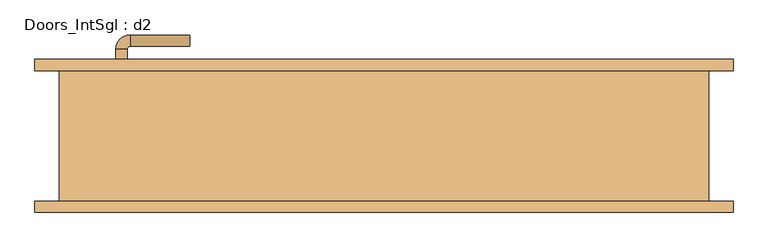
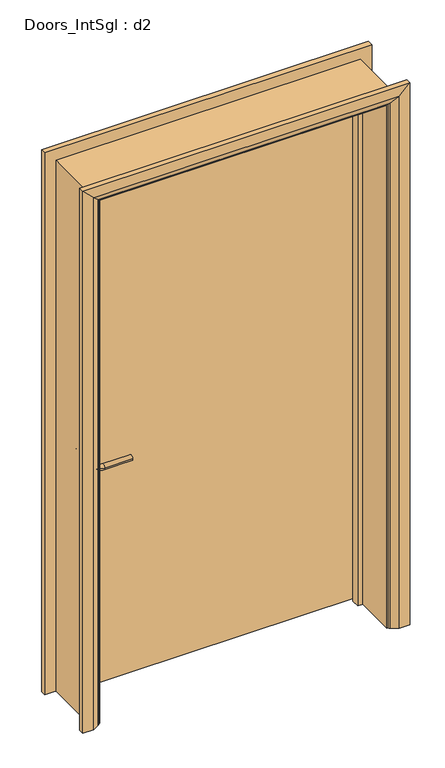
"""IFC4 building model written with IfcOpenShell, lengths in millimetres: door geometry, Doors_IntSgl : d2."""

from ifc_helpers import new_model, si_unit, point, frame, frame_2d, origin, place, context, project, spatial, polyline, circle_curve, ellipse_curve, trimmed, segment, composite_curve, outline, extrude, faceted_brep, source, transform, mapped, element, save
from ifc_brep_helpers import plane_surface, cylinder_surface, revolved_surface, advanced_brep


def doors_intsgl_d2_d6dd0e7a(model_context):
    return source(origin(), model_context, "Body", "SolidModel", [
        advanced_brep(
        [(-470.85, 68.3, 900.0), (-450.85, 68.3, 900.0), (-450.85, 38.3, 900.0), (-470.85, 38.3, 900.0), (-445.85, 33.3, 900.0), (-445.85, 13.3, 900.0), (-340.85, 13.3, 900.0), (-340.85, 33.3, 900.0)],
        [
            (0, 1, circle_curve(frame((-460.85, 68.3, 900.0), z_axis=(0.0, 1.0, 0.0), x_axis=(1.0, 0.0, 0.0)), 10.0)),
            (1, 0, circle_curve(frame((-460.85, 68.3, 900.0), z_axis=(0.0, 1.0, 0.0), x_axis=(1.0, 0.0, 0.0)), 10.0)),
            (1, 2),
            (2, 3, circle_curve(frame((-460.85, 38.3, 900.0), z_axis=(0.0, 1.0, 0.0), x_axis=(1.0, 0.0, 0.0)), 10.0)),
            (3, 0),
            (3, 2, circle_curve(frame((-460.85, 38.3, 900.0), z_axis=(0.0, 1.0, 0.0), x_axis=(1.0, 0.0, 0.0)), 10.0)),
            (4, 5, circle_curve(frame((-445.85, 23.3, 900.0), z_axis=(-1.0, 0.0, 0.0), x_axis=(0.0, 1.0, 0.0)), 10.0)),
            (5, 3, circle_curve(frame((-445.85, 38.3, 900.0), z_axis=(0.0, 0.0, -1.0), x_axis=(-1.0, 0.0, 0.0)), 25.0)),
            (2, 4, circle_curve(frame((-445.85, 38.3, 900.0), z_axis=(0.0, 0.0, 1.0), x_axis=(-1.0, 0.0, 0.0)), 5.0)),
            (5, 4, circle_curve(frame((-445.85, 23.3, 900.0), z_axis=(-1.0, 0.0, 0.0), x_axis=(0.0, 1.0, 0.0)), 10.0)),
            (6, 7, circle_curve(frame((-340.85, 23.3, 900.0), z_axis=(1.0, 0.0, 0.0), x_axis=(0.0, 1.0, 0.0)), 10.0)),
            (7, 6, circle_curve(frame((-340.85, 23.3, 900.0), z_axis=(1.0, 0.0, 0.0), x_axis=(0.0, 1.0, 0.0)), 10.0)),
            (4, 7),
            (6, 5),
        ],
        [
            plane_surface(frame((-460.85, 68.3, 900.0), z_axis=(0.0, 1.0, 0.0), x_axis=(0.0, 0.0, 1.0))),
            cylinder_surface(frame((-460.85, 68.3, 900.0), z_axis=(0.0, 1.0, 0.0), x_axis=(1.0, 0.0, 0.0)), 10.0),
            revolved_surface(trimmed(ellipse_curve(frame((-460.85, 38.3, 900.0), z_axis=(0.0, -1.0, 0.0), x_axis=(1.0, 0.0, 0.0)), 10.0, 10.0), [point((-470.85, 38.3, 900.0))], [point((-450.85, 38.3, 900.0))], True, "CARTESIAN"), (-445.85, 38.3, 900.0), (0.0, 0.0, -1.0)),
            revolved_surface(trimmed(ellipse_curve(frame((-460.85, 38.3, 900.0), z_axis=(0.0, -1.0, 0.0), x_axis=(1.0, 0.0, 0.0)), 10.0, 10.0), [point((-450.85, 38.3, 900.0))], [point((-470.85, 38.3, 900.0))], True, "CARTESIAN"), (-445.85, 38.3, 900.0), (0.0, 0.0, -1.0)),
            plane_surface(frame((-340.85, 23.3, 900.0), z_axis=(1.0, 0.0, 0.0), x_axis=(0.0, 0.0, 1.0))),
            cylinder_surface(frame((-445.85, 23.3, 900.0), z_axis=(-1.0, 0.0, 0.0), x_axis=(0.0, 1.0, 0.0)), 10.0),
        ],
        [
            (0, [[1, 2]]),
            (1, [[3, 4, 5, -2]]),
            (1, [[-5, 6, -3, -1]]),
            (2, [[7, 8, -4, 9]]),
            (3, [[10, -9, -6, -8]]),
            (4, [[11, 12]]),
            (5, [[13, -11, 14, -7]]),
            (5, [[-14, -12, -13, -10]]),
        ],
    ),
        extrude(outline(composite_curve([segment(trimmed(circle_curve(frame_2d((900.0, -463.35)), 30.0), [point((900.0, -493.35))], [point((900.0, -433.35))], False, "CARTESIAN"), True, "CONTINUOUS"), segment(trimmed(circle_curve(frame_2d((900.0, -463.35)), 30.0), [point((900.0, -433.35))], [point((900.0, -493.35))], False, "CARTESIAN"), True, "CONTINUOUS")], self_intersect=False)), frame((0.0, 68.3, 0.0), z_axis=(0.0, 1.0, 0.0), x_axis=(0.0, 0.0, 1.0)), (0.0, 0.0, 1.0), 8.0),
        advanced_brep(
        [(-470.85, 122.3, 900.0), (-450.85, 122.3, 900.0), (-470.85, 152.3, 900.0), (-450.85, 152.3, 900.0), (-445.85, 157.3, 900.0), (-445.85, 177.3, 900.0), (-340.85, 177.3, 900.0), (-340.85, 157.3, 900.0)],
        [
            (0, 1, circle_curve(frame((-460.85, 122.3, 900.0), z_axis=(0.0, -1.0, 0.0), x_axis=(1.0, 0.0, 0.0)), 10.0)),
            (1, 0, circle_curve(frame((-460.85, 122.3, 900.0), z_axis=(0.0, -1.0, 0.0), x_axis=(1.0, 0.0, 0.0)), 10.0)),
            (0, 2),
            (2, 3, circle_curve(frame((-460.85, 152.3, 900.0), z_axis=(0.0, -1.0, 0.0), x_axis=(1.0, 0.0, 0.0)), 10.0)),
            (3, 1),
            (3, 2, circle_curve(frame((-460.85, 152.3, 900.0), z_axis=(0.0, -1.0, 0.0), x_axis=(1.0, 0.0, 0.0)), 10.0)),
            (4, 3, circle_curve(frame((-445.85, 152.3, 900.0), z_axis=(0.0, 0.0, 1.0), x_axis=(-1.0, 0.0, 0.0)), 5.0)),
            (2, 5, circle_curve(frame((-445.85, 152.3, 900.0), z_axis=(0.0, 0.0, -1.0), x_axis=(-1.0, 0.0, 0.0)), 25.0)),
            (5, 4, circle_curve(frame((-445.85, 167.3, 900.0), z_axis=(-1.0, 0.0, 0.0), x_axis=(0.0, -1.0, 0.0)), 10.0)),
            (4, 5, circle_curve(frame((-445.85, 167.3, 900.0), z_axis=(-1.0, 0.0, 0.0), x_axis=(0.0, -1.0, 0.0)), 10.0)),
            (6, 7, circle_curve(frame((-340.85, 167.3, 900.0), z_axis=(1.0, 0.0, 0.0), x_axis=(0.0, -1.0, 0.0)), 10.0)),
            (7, 6, circle_curve(frame((-340.85, 167.3, 900.0), z_axis=(1.0, 0.0, 0.0), x_axis=(0.0, -1.0, 0.0)), 10.0)),
            (5, 6),
            (7, 4),
        ],
        [
            plane_surface(frame((-460.85, 122.3, 900.0), z_axis=(0.0, -1.0, 0.0), x_axis=(0.0, 0.0, 1.0))),
            cylinder_surface(frame((-460.85, 122.3, 900.0), z_axis=(0.0, -1.0, 0.0), x_axis=(1.0, 0.0, 0.0)), 10.0),
            revolved_surface(trimmed(ellipse_curve(frame((-460.85, 152.3, 900.0), z_axis=(0.0, -1.0, 0.0), x_axis=(1.0, 0.0, 0.0)), 10.0, 10.0), [point((-470.85, 152.3, 900.0))], [point((-450.85, 152.3, 900.0))], True, "CARTESIAN"), (-445.85, 152.3, 900.0), (0.0, 0.0, -1.0)),
            revolved_surface(trimmed(ellipse_curve(frame((-460.85, 152.3, 900.0), z_axis=(0.0, -1.0, 0.0), x_axis=(1.0, 0.0, 0.0)), 10.0, 10.0), [point((-450.85, 152.3, 900.0))], [point((-470.85, 152.3, 900.0))], True, "CARTESIAN"), (-445.85, 152.3, 900.0), (0.0, 0.0, -1.0)),
            plane_surface(frame((-340.85, 167.3, 900.0), z_axis=(1.0, 0.0, 0.0), x_axis=(0.0, 0.0, 1.0))),
            cylinder_surface(frame((-445.85, 167.3, 900.0), z_axis=(-1.0, 0.0, 0.0), x_axis=(0.0, -1.0, 0.0)), 10.0),
        ],
        [
            (0, [[1, 2]]),
            (1, [[-1, 3, 4, 5]]),
            (1, [[-2, -5, 6, -3]]),
            (2, [[7, -4, 8, 9]]),
            (3, [[-8, -6, -7, 10]]),
            (4, [[11, 12]]),
            (5, [[-9, 13, -12, 14]]),
            (5, [[-10, -14, -11, -13]]),
        ],
    ),
        extrude(outline(composite_curve([segment(trimmed(circle_curve(frame_2d((900.0, -463.35)), 30.0), [point((900.0, -493.35))], [point((900.0, -433.35))], False, "CARTESIAN"), True, "CONTINUOUS"), segment(trimmed(circle_curve(frame_2d((900.0, -463.35)), 30.0), [point((900.0, -433.35))], [point((900.0, -493.35))], False, "CARTESIAN"), True, "CONTINUOUS")], self_intersect=False)), frame((0.0, 114.3, 0.0), z_axis=(0.0, 1.0, 0.0), x_axis=(0.0, 0.0, 1.0)), (0.0, 0.0, 1.0), 8.0),
        extrude(outline(polyline([(535.85, 76.3), (-535.85, 76.3), (-535.85, 114.3), (535.85, 114.3), (535.85, 76.3)])), frame((0.0, 0.0, 8.0), z_axis=(0.0, 0.0, 1.0), x_axis=(1.0, 0.0, 0.0)), (0.0, 0.0, 1.0), 2060.0),
        advanced_brep(
        [(612.85, 134.3, 0.0), (612.85, 114.3, 0.0), (542.85, 114.3, 0.0), (546.85, 120.3, 0.0), (572.85, 134.3, 0.0), (612.85, 134.3, 2145.0), (612.85, 114.3, 2145.0), (-612.85, 114.3, 2145.0), (-612.85, 114.3, 0.0), (-542.85, 114.3, 0.0), (-542.85, 114.3, 2075.0), (542.85, 114.3, 2075.0), (546.85, 120.3, 2079.0), (572.85, 134.3, 2105.0), (-572.85, 134.3, 2105.0), (-572.85, 134.3, 0.0), (-612.85, 134.3, 0.0), (-612.85, 134.3, 2145.0), (-546.85, 120.3, 0.0), (-546.85, 120.3, 2079.0)],
        [
            (0, 1),
            (1, 2),
            (2, 3, circle_curve(frame((550.85, 113.3, 0.0), z_axis=(0.0, 0.0, -1.0), x_axis=(1.0, 0.0, 0.0)), 8.0622577)),
            (3, 4),
            (4, 0),
            (0, 5),
            (5, 6),
            (6, 1),
            (6, 7),
            (7, 8),
            (8, 9),
            (9, 10),
            (10, 11),
            (11, 2),
            (11, 12, ellipse_curve(frame((550.85, 113.3, 2083.0), z_axis=(0.7071067811865475, 0.0, -0.7071067811865475), x_axis=(-0.7071067811865474, 0.0, -0.7071067811865476)), 11.4017543, 8.0622577)),
            (12, 3),
            (12, 13),
            (13, 4),
            (13, 14),
            (14, 15),
            (15, 16),
            (16, 17),
            (17, 5),
            (7, 17),
            (16, 8),
            (15, 18),
            (18, 9, circle_curve(frame((-550.85, 113.3, 0.0), z_axis=(0.0, 0.0, -1.0), x_axis=(-1.0, 0.0, 0.0)), 8.0622577)),
            (19, 10, ellipse_curve(frame((-550.85, 113.3, 2083.0), z_axis=(-0.7071067811865475, 0.0, -0.7071067811865475), x_axis=(-0.7071067811865474, 0.0, 0.7071067811865476)), 11.4017543, 8.0622577)),
            (18, 19),
            (14, 19),
            (19, 12),
        ],
        [
            plane_surface(frame((542.85, 114.3, 0.0), z_axis=(0.0, 0.0, -1.0), x_axis=(0.0, -1.0, 0.0))),
            plane_surface(frame((612.85, 134.3, 0.0), z_axis=(1.0, 0.0, 0.0), x_axis=(0.0, 0.0, 1.0))),
            plane_surface(frame((612.85, 114.3, 0.0), z_axis=(0.0, -1.0, 0.0), x_axis=(0.0, 0.0, 1.0))),
            cylinder_surface(frame((550.85, 113.3, 0.0), z_axis=(0.0, 0.0, -1.0), x_axis=(1.0, 0.0, 0.0)), 8.0622577),
            plane_surface(frame((546.85, 120.3, 0.0), z_axis=(-0.4740998230350126, 0.880471099922178, 0.0), x_axis=(0.0, 0.0, 1.0))),
            plane_surface(frame((572.85, 134.3, 0.0), z_axis=(0.0, 1.0, 0.0), x_axis=(0.0, 0.0, 1.0))),
            plane_surface(frame((-612.85, 134.3, 2145.0), z_axis=(-1.0, 0.0, 0.0), x_axis=(0.0, 0.0, -1.0))),
            plane_surface(frame((-542.85, 114.3, 0.0), z_axis=(0.0, 0.0, -1.0), x_axis=(0.0, -1.0, 0.0))),
            cylinder_surface(frame((-550.85, 113.3, 2075.0), z_axis=(0.0, 0.0, 1.0), x_axis=(-1.0, 0.0, 0.0)), 8.0622577),
            plane_surface(frame((-546.85, 120.3, 2079.0), z_axis=(0.47409982303501824, 0.8804710999221749, 0.0), x_axis=(0.0, 0.0, -1.0))),
            plane_surface(frame((612.85, 134.3, 2145.0), z_axis=(0.0, 0.0, 1.0), x_axis=(-1.0, 0.0, 0.0))),
            cylinder_surface(frame((542.85, 113.3, 2083.0), z_axis=(1.0, 0.0, 0.0), x_axis=(0.0, 0.0, 1.0)), 8.0622577),
            plane_surface(frame((546.85, 120.3, 2079.0), z_axis=(0.0, 0.8804710999221764, -0.4740998230350154), x_axis=(-1.0, 0.0, 0.0))),
        ],
        [
            (0, [[1, 2, 3, 4, 5]]),
            (1, [[-1, 6, 7, 8]]),
            (2, [[-2, -8, 9, 10, 11, 12, 13, 14]]),
            (3, [[-3, -14, 15, 16]]),
            (4, [[-4, -16, 17, 18]]),
            (5, [[-5, -18, 19, 20, 21, 22, 23, -6]]),
            (6, [[24, -22, 25, -10]]),
            (7, [[-21, 26, 27, -11, -25]]),
            (8, [[28, -12, -27, 29]]),
            (9, [[30, -29, -26, -20]]),
            (10, [[-7, -23, -24, -9]]),
            (11, [[-15, -13, -28, 31]]),
            (12, [[-17, -31, -30, -19]]),
        ],
    ),
        extrude(outline(polyline([(0.0, -537.85), (0.0, -518.85), (2051.0, -518.85), (2051.0, 518.85), (0.0, 518.85), (0.0, 537.85), (2070.0, 537.85), (2070.0, -537.85), (0.0, -537.85)])), frame((0.0, 42.3, 0.0), z_axis=(0.0, 1.0, 0.0), x_axis=(0.0, 0.0, 1.0)), (0.0, 0.0, 1.0), 32.0),
        advanced_brep(
        [(-612.85, -134.3, 0.0), (-612.85, -114.3, 0.0), (-542.85, -114.3, 0.0), (-546.85, -120.3, 0.0), (-572.85, -134.3, 0.0), (-612.85, -134.3, 2145.0), (-612.85, -114.3, 2145.0), (-542.85, -114.3, 2075.0), (-546.85, -120.3, 2079.0), (-572.85, -134.3, 2105.0), (612.85, -134.3, 0.0), (572.85, -134.3, 0.0), (546.85, -120.3, 0.0), (542.85, -114.3, 0.0), (612.85, -114.3, 0.0), (612.85, -134.3, 2145.0), (572.85, -134.3, 2105.0), (546.85, -120.3, 2079.0), (542.85, -114.3, 2075.0), (612.85, -114.3, 2145.0)],
        [
            (0, 1),
            (1, 2),
            (2, 3, circle_curve(frame((-550.85, -113.3, 0.0), z_axis=(0.0, 0.0, -1.0), x_axis=(-1.0, 0.0, 0.0)), 8.0622577)),
            (3, 4),
            (4, 0),
            (0, 5),
            (5, 6),
            (6, 1),
            (6, 7),
            (7, 2),
            (7, 8, ellipse_curve(frame((-550.85, -113.3, 2083.0), z_axis=(-0.7071067811865475, 0.0, -0.7071067811865475), x_axis=(0.7071067811865474, 0.0, -0.7071067811865476)), 11.4017543, 8.0622577)),
            (8, 3),
            (8, 9),
            (9, 4),
            (9, 5),
            (10, 11),
            (11, 12),
            (12, 13, circle_curve(frame((550.85, -113.3, 0.0), z_axis=(0.0, 0.0, -1.0), x_axis=(1.0, 0.0, 0.0)), 8.0622577)),
            (13, 14),
            (14, 10),
            (15, 16),
            (16, 11),
            (10, 15),
            (16, 17),
            (17, 12),
            (17, 18, ellipse_curve(frame((550.85, -113.3, 2083.0), z_axis=(0.7071067811865475, 0.0, -0.7071067811865475), x_axis=(0.7071067811865474, 0.0, 0.7071067811865476)), 11.4017543, 8.0622577)),
            (18, 13),
            (18, 19),
            (19, 14),
            (19, 15),
            (5, 15),
            (19, 6),
            (18, 7),
            (17, 8),
            (16, 9),
        ],
        [
            plane_surface(frame((-542.85, -187.1010989, 0.0), z_axis=(0.0, 0.0, -1.0), x_axis=(1.0, 0.0, 0.0))),
            plane_surface(frame((-612.85, -134.3, 0.0), z_axis=(-1.0, 0.0, 0.0), x_axis=(0.0, 0.0, 1.0))),
            plane_surface(frame((-612.85, -114.3, 0.0), z_axis=(0.0, 1.0, 0.0), x_axis=(0.0, 0.0, 1.0))),
            cylinder_surface(frame((-550.85, -113.3, 0.0), z_axis=(0.0, 0.0, -1.0), x_axis=(-1.0, 0.0, 0.0)), 8.0622577),
            plane_surface(frame((-546.85, -120.3, 0.0), z_axis=(0.4740998230350183, -0.8804710999221749, 0.0), x_axis=(0.0, 0.0, 1.0))),
            plane_surface(frame((-572.85, -134.3, 0.0), z_axis=(0.0, -1.0, 0.0), x_axis=(0.0, 0.0, 1.0))),
            plane_surface(frame((542.85, -187.1010989, 0.0), z_axis=(0.0, 0.0, -1.0), x_axis=(-1.0, 0.0, 0.0))),
            plane_surface(frame((572.85, -134.3, 2105.0), z_axis=(0.0, -1.0, 0.0), x_axis=(0.0, 0.0, -1.0))),
            plane_surface(frame((546.85, -120.3, 2079.0), z_axis=(-0.4740998230350183, -0.8804710999221749, 0.0), x_axis=(0.0, 0.0, -1.0))),
            cylinder_surface(frame((550.85, -113.3, 2075.0), z_axis=(0.0, 0.0, 1.0), x_axis=(1.0, 0.0, 0.0)), 8.0622577),
            plane_surface(frame((612.85, -114.3, 2145.0), z_axis=(0.0, 1.0, 0.0), x_axis=(0.0, 0.0, -1.0))),
            plane_surface(frame((612.85, -134.3, 2145.0), z_axis=(1.0, 0.0, 0.0), x_axis=(0.0, 0.0, -1.0))),
            plane_surface(frame((-612.85, -134.3, 2145.0), z_axis=(0.0, 0.0, 1.0), x_axis=(1.0, 0.0, 0.0))),
            plane_surface(frame((-612.85, -114.3, 2145.0), z_axis=(0.0, 1.0, 0.0), x_axis=(1.0, 0.0, 0.0))),
            cylinder_surface(frame((-542.85, -113.3, 2083.0), z_axis=(-1.0, 0.0, 0.0), x_axis=(0.0, 0.0, 1.0)), 8.0622577),
            plane_surface(frame((-546.85, -120.3, 2079.0), z_axis=(0.0, -0.8804710999221749, -0.4740998230350183), x_axis=(1.0, 0.0, 0.0))),
            plane_surface(frame((-572.85, -134.3, 2105.0), z_axis=(0.0, -1.0, 0.0), x_axis=(1.0, 0.0, 0.0))),
        ],
        [
            (0, [[1, 2, 3, 4, 5]]),
            (1, [[-1, 6, 7, 8]]),
            (2, [[-2, -8, 9, 10]]),
            (3, [[-3, -10, 11, 12]]),
            (4, [[-4, -12, 13, 14]]),
            (5, [[-5, -14, 15, -6]]),
            (6, [[16, 17, 18, 19, 20]]),
            (7, [[21, 22, -16, 23]]),
            (8, [[24, 25, -17, -22]]),
            (9, [[26, 27, -18, -25]]),
            (10, [[28, 29, -19, -27]]),
            (11, [[30, -23, -20, -29]]),
            (12, [[-7, 31, -30, 32]]),
            (13, [[-9, -32, -28, 33]]),
            (14, [[-11, -33, -26, 34]]),
            (15, [[-13, -34, -24, 35]]),
            (16, [[-15, -35, -21, -31]]),
        ],
    ),
        faceted_brep([(-537.85, 114.3, 0.0), (-537.85, -114.3, 0.0), (-569.85, -114.3, 0.0), (-569.85, 114.3, 0.0), (-537.85, 114.3, 2070.0), (-537.85, -114.3, 2070.0), (-569.85, -114.3, 2102.0), (-569.85, 114.3, 2102.0), (537.85, 114.3, 0.0), (569.85, 114.3, 0.0), (569.85, -114.3, 0.0), (537.85, -114.3, 0.0), (537.85, 114.3, 2070.0), (569.85, 114.3, 2102.0), (569.85, -114.3, 2102.0), (537.85, -114.3, 2070.0)], [[[0, 1, 2, 3]], [[1, 0, 4, 5]], [[2, 1, 5, 6]], [[3, 2, 6, 7]], [[0, 3, 7, 4]], [[8, 9, 10, 11]], [[12, 13, 9, 8]], [[13, 14, 10, 9]], [[14, 15, 11, 10]], [[15, 12, 8, 11]], [[5, 4, 12, 15]], [[6, 5, 15, 14]], [[7, 6, 14, 13]], [[4, 7, 13, 12]]]),
    ])


if __name__ == "__main__":
    model = new_model("IFC4")
    model_context = context("Model", 3, world=origin())
    ifc_project = project(units=[si_unit("LENGTHUNIT", "METRE", prefix="MILLI")], contexts=[model_context])
    site = spatial("IfcSite", under=ifc_project)
    building = spatial("IfcBuilding", under=site)
    placement = place(None, origin())
    doors_intsgl_d2_shape = doors_intsgl_d2_d6dd0e7a(model_context)
    element("IfcDoor", 1, ObjectType="Doors_IntSgl : d2", at=placement, inside=building, context=model_context, shape_type="MappedRepresentation", body=[
        mapped(doors_intsgl_d2_shape, transform((0.0, 0.0, 0.0), x_axis=(1.0, 0.0, 0.0), y_axis=(0.0, 1.0, 0.0), z_axis=(0.0, 0.0, 1.0))),
    ])
    save(model, "model.ifc")

# Revit data of these elements
# Type "Doors_IntSgl : d2"
#   Type Mark = "48"
#   Type Comments = "Internal Single"
#   Operation = "SingleSwingRight"
#   Manufacturer = "Revit"
#   Keynote = "L20"
#   Description = "Internal Single Door"
#   Analytic Construction = "Metal"
#   UnderCut = 0' - 0.31496"
#   Tolerance = 0' - 0.07874"
#   Thickness = 0' - 1.49606"
#   Thermal Resistance (R) = 0.270117 (m²·K)/W
#   Structural Tolerance = 0' - 0.31496"
#   StopDepth = 0' - 1.25984"
#   Stop Thickness = 0' - 0.74803"
#   Rough Width = 3' - 9 1/2"
#   Rough Height = 6' - 11.07087"
#   Height to Top Lock Rail = 3' - 3.37008"
#   Heat Transfer Coefficient (U) = 3.7021 W/(m²·K)
#   Handle Z Distance = 2' - 11.43307"
#   Handle X Distance = 0' - 2.95276"
#   Frame Thickness = 0' - 1.25984"
#   Door Panel Width = 3' - 6.19291"
#   Door Panel Thickness = 0' - 1.49606"
#   Door Panel Offset = 0' - 0"
#   Height = 6' - 11.07087"
#   Width = 3' - 9 1/2"
#   Door Panel Height = 6' - 9.10236"
#   Architrave Setback = 0' - 0.19685"
#   Vis - Ironmongery = yes
#   Material Ironmongery = Door - Handle
#   Material Frame = Door - Frame/Mullion (1)
#   Material Door = Door - Panel
#   Material Architrave = Door - Architrave
#   Visual Light Transmittance = 0
#   Solar Heat Gain Coefficient = 0
#   Function = (empty or 0)
#   Wall Closure = (empty or 0)
# Element 1 (IfcDoor, "Doors_IntSgl : d2")
#   Materials on its faces: "Door - Architrave", "Door - Handle", "Door - Frame/Mullion (1)", "Door - Panel"
# Materials
#   "Door - Handle": colour RGB 0 0 0, transparency 0, Keynote = "P21", Cost = 0
#   "Door - Frame/Mullion (1)": class "Wood", colour RGB 212 179 113, transparency 0, Keynote = "L20", Cost = 0
#   "Door - Panel": class "Wood", colour RGB 210 159 95, transparency 0, Keynote = "L20", Cost = 0
#   "Door - Architrave": class "Wood", colour RGB 154 90 5, transparency 0, Keynote = "P20", Cost = 0
